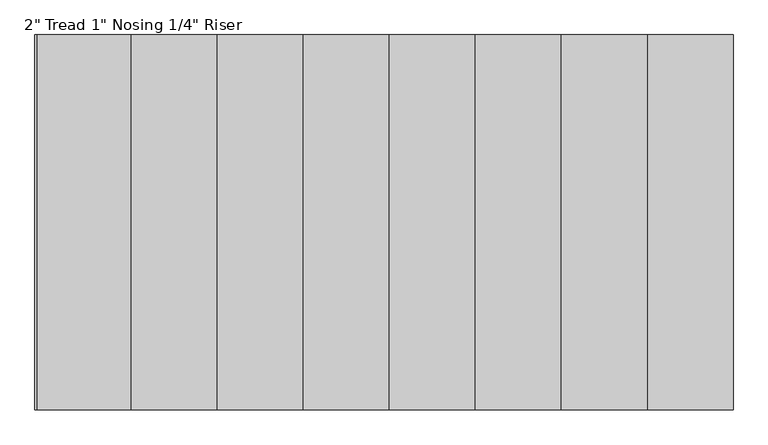
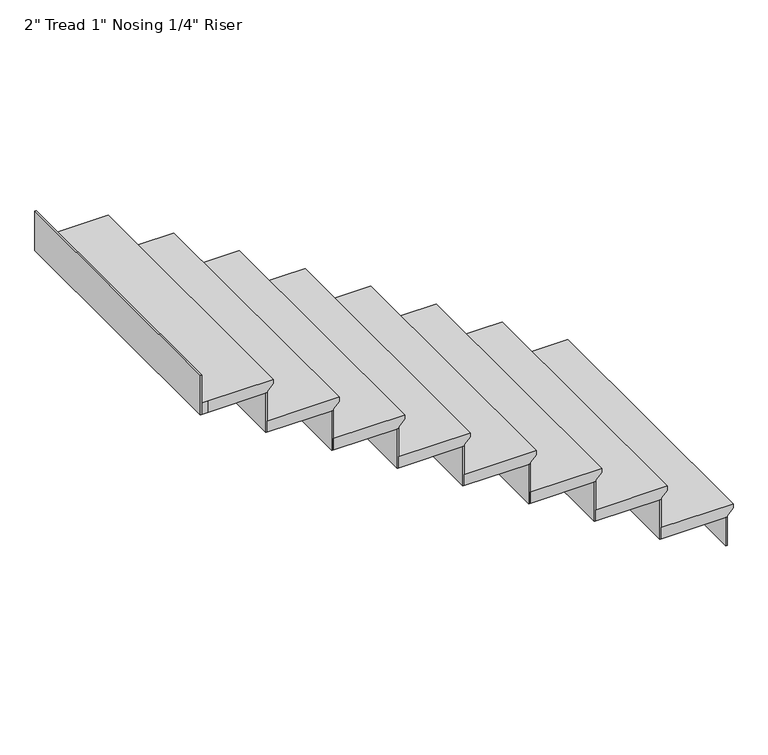
"""IFC4 building model written with IfcOpenShell, lengths in millimetres: stair flight geometry."""

from ifc_helpers import new_model, si_unit, origin, place, context, project, spatial, faceted_brep, source, transform, mapped, element, save


def stair_flight_d31f5684(model_context):
    return source(origin(), model_context, "Body", "Brep", [
        faceted_brep([(-5888.2707895, 6233.3144188, 3359.15), (-5888.2707895, 6233.3144188, 3378.2), (-5888.2707895, 5014.1144188, 3378.2), (-5888.2707895, 5014.1144188, 3359.15), (-5913.6707895, 6233.3144188, 3333.75), (-5913.6707895, 5014.1144188, 3333.75), (-6193.0707895, 6233.3144188, 3378.2), (-6193.0707895, 5014.1144188, 3378.2), (-5913.6707895, 5014.1144188, 3327.4), (-6193.0707895, 5014.1144188, 3327.4), (-6193.0707895, 6233.3144188, 3327.4), (-5913.6707895, 6233.3144188, 3327.4)], [[[0, 1, 2, 3]], [[4, 0, 3, 5]], [[2, 1, 6, 7]], [[8, 9, 10, 11]], [[2, 7, 9, 8, 5, 3]], [[8, 11, 4, 5]], [[6, 1, 0, 4, 11, 10]], [[7, 6, 10, 9]]]),
        faceted_brep([(-5913.6707895, 6233.3144188, 3327.4), (-5913.6707895, 6233.3144188, 3200.4), (-5920.0207895, 6233.3144188, 3200.4), (-5920.0207895, 6233.3144188, 3327.4), (-5913.6707895, 5014.1144188, 3327.4), (-5920.0207895, 5014.1144188, 3327.4), (-5920.0207895, 5014.1144188, 3200.4), (-5913.6707895, 5014.1144188, 3200.4)], [[[0, 1, 2, 3]], [[4, 5, 6, 7]], [[1, 0, 4, 7]], [[2, 1, 7, 6]], [[3, 2, 6, 5]], [[0, 3, 5, 4]]]),
        faceted_brep([(-6193.0707895, 6233.3144188, 3505.2), (-6193.0707895, 6233.3144188, 3327.4), (-6199.4207895, 6233.3144188, 3327.4), (-6199.4207895, 6233.3144188, 3505.2), (-6193.0707895, 5014.1144188, 3505.2), (-6199.4207895, 5014.1144188, 3505.2), (-6199.4207895, 5014.1144188, 3327.4), (-6193.0707895, 5014.1144188, 3327.4)], [[[0, 1, 2, 3]], [[4, 5, 6, 7]], [[1, 0, 4, 7]], [[2, 1, 7, 6]], [[3, 2, 6, 5]], [[0, 3, 5, 4]]]),
        faceted_brep([(-6167.6707895, 5014.1144188, 3556.0), (-6167.6707895, 6233.3144188, 3556.0), (-6472.4707895, 6233.3144188, 3556.0), (-6472.4707895, 5014.1144188, 3556.0), (-6193.0707895, 5014.1144188, 3505.2), (-6472.4707895, 5014.1144188, 3505.2), (-6472.4707895, 6233.3144188, 3505.2), (-6193.0707895, 6233.3144188, 3505.2), (-6193.0707895, 5014.1144188, 3511.55), (-6167.6707895, 5014.1144188, 3536.95), (-6193.0707895, 6233.3144188, 3511.55), (-6167.6707895, 6233.3144188, 3536.95)], [[[0, 1, 2, 3]], [[4, 5, 6, 7]], [[0, 3, 5, 4, 8, 9]], [[4, 7, 10, 8]], [[2, 1, 11, 10, 7, 6]], [[3, 2, 6, 5]], [[11, 1, 0, 9]], [[10, 11, 9, 8]]]),
        faceted_brep([(-6472.4707895, 6233.3144188, 3683.0), (-6472.4707895, 6233.3144188, 3505.2), (-6478.8207895, 6233.3144188, 3505.2), (-6478.8207895, 6233.3144188, 3683.0), (-6472.4707895, 5014.1144188, 3683.0), (-6478.8207895, 5014.1144188, 3683.0), (-6478.8207895, 5014.1144188, 3505.2), (-6472.4707895, 5014.1144188, 3505.2)], [[[0, 1, 2, 3]], [[4, 5, 6, 7]], [[1, 0, 4, 7]], [[2, 1, 7, 6]], [[3, 2, 6, 5]], [[0, 3, 5, 4]]]),
        faceted_brep([(-6447.0707895, 5014.1144188, 3733.8), (-6447.0707895, 6233.3144188, 3733.8), (-6751.8707895, 6233.3144188, 3733.8), (-6751.8707895, 5014.1144188, 3733.8), (-6472.4707895, 5014.1144188, 3683.0), (-6751.8707895, 5014.1144188, 3683.0), (-6751.8707895, 6233.3144188, 3683.0), (-6472.4707895, 6233.3144188, 3683.0), (-6472.4707895, 5014.1144188, 3689.35), (-6447.0707895, 5014.1144188, 3714.75), (-6472.4707895, 6233.3144188, 3689.35), (-6447.0707895, 6233.3144188, 3714.75)], [[[0, 1, 2, 3]], [[4, 5, 6, 7]], [[0, 3, 5, 4, 8, 9]], [[4, 7, 10, 8]], [[2, 1, 11, 10, 7, 6]], [[3, 2, 6, 5]], [[11, 1, 0, 9]], [[10, 11, 9, 8]]]),
        faceted_brep([(-6751.8707895, 6233.3144188, 3860.8), (-6751.8707895, 6233.3144188, 3683.0), (-6758.2207895, 6233.3144188, 3683.0), (-6758.2207895, 6233.3144188, 3860.8), (-6751.8707895, 5014.1144188, 3860.8), (-6758.2207895, 5014.1144188, 3860.8), (-6758.2207895, 5014.1144188, 3683.0), (-6751.8707895, 5014.1144188, 3683.0)], [[[0, 1, 2, 3]], [[4, 5, 6, 7]], [[1, 0, 4, 7]], [[2, 1, 7, 6]], [[3, 2, 6, 5]], [[0, 3, 5, 4]]]),
        faceted_brep([(-6726.4707895, 5014.1144188, 3911.6), (-6726.4707895, 6233.3144188, 3911.6), (-7031.2707895, 6233.3144188, 3911.6), (-7031.2707895, 5014.1144188, 3911.6), (-6751.8707895, 5014.1144188, 3860.8), (-7031.2707895, 5014.1144188, 3860.8), (-7031.2707895, 6233.3144188, 3860.8), (-6751.8707895, 6233.3144188, 3860.8), (-6751.8707895, 5014.1144188, 3867.15), (-6726.4707895, 5014.1144188, 3892.55), (-6751.8707895, 6233.3144188, 3867.15), (-6726.4707895, 6233.3144188, 3892.55)], [[[0, 1, 2, 3]], [[4, 5, 6, 7]], [[0, 3, 5, 4, 8, 9]], [[4, 7, 10, 8]], [[2, 1, 11, 10, 7, 6]], [[3, 2, 6, 5]], [[11, 1, 0, 9]], [[10, 11, 9, 8]]]),
        faceted_brep([(-7031.2707895, 6233.3144188, 4038.6), (-7031.2707895, 6233.3144188, 3860.8), (-7037.6207895, 6233.3144188, 3860.8), (-7037.6207895, 6233.3144188, 4038.6), (-7031.2707895, 5014.1144188, 4038.6), (-7037.6207895, 5014.1144188, 4038.6), (-7037.6207895, 5014.1144188, 3860.8), (-7031.2707895, 5014.1144188, 3860.8)], [[[0, 1, 2, 3]], [[4, 5, 6, 7]], [[1, 0, 4, 7]], [[2, 1, 7, 6]], [[3, 2, 6, 5]], [[0, 3, 5, 4]]]),
        faceted_brep([(-7005.8707895, 5014.1144188, 4089.4), (-7005.8707895, 6233.3144188, 4089.4), (-7310.6707895, 6233.3144188, 4089.4), (-7310.6707895, 5014.1144188, 4089.4), (-7031.2707895, 5014.1144188, 4038.6), (-7310.6707895, 5014.1144188, 4038.6), (-7310.6707895, 6233.3144188, 4038.6), (-7031.2707895, 6233.3144188, 4038.6), (-7031.2707895, 5014.1144188, 4044.95), (-7005.8707895, 5014.1144188, 4070.35), (-7031.2707895, 6233.3144188, 4044.95), (-7005.8707895, 6233.3144188, 4070.35)], [[[0, 1, 2, 3]], [[4, 5, 6, 7]], [[0, 3, 5, 4, 8, 9]], [[4, 7, 10, 8]], [[2, 1, 11, 10, 7, 6]], [[3, 2, 6, 5]], [[11, 1, 0, 9]], [[10, 11, 9, 8]]]),
        faceted_brep([(-7310.6707895, 6233.3144188, 4216.4), (-7310.6707895, 6233.3144188, 4038.6), (-7317.0207895, 6233.3144188, 4038.6), (-7317.0207895, 6233.3144188, 4216.4), (-7310.6707895, 5014.1144188, 4216.4), (-7317.0207895, 5014.1144188, 4216.4), (-7317.0207895, 5014.1144188, 4038.6), (-7310.6707895, 5014.1144188, 4038.6)], [[[0, 1, 2, 3]], [[4, 5, 6, 7]], [[1, 0, 4, 7]], [[2, 1, 7, 6]], [[3, 2, 6, 5]], [[0, 3, 5, 4]]]),
        faceted_brep([(-7285.2707895, 5014.1144188, 4267.2), (-7285.2707895, 6233.3144188, 4267.2), (-7590.0707895, 6233.3144188, 4267.2), (-7590.0707895, 5014.1144188, 4267.2), (-7310.6707895, 5014.1144188, 4216.4), (-7590.0707895, 5014.1144188, 4216.4), (-7590.0707895, 6233.3144188, 4216.4), (-7310.6707895, 6233.3144188, 4216.4), (-7310.6707895, 5014.1144188, 4222.75), (-7285.2707895, 5014.1144188, 4248.15), (-7310.6707895, 6233.3144188, 4222.75), (-7285.2707895, 6233.3144188, 4248.15)], [[[0, 1, 2, 3]], [[4, 5, 6, 7]], [[0, 3, 5, 4, 8, 9]], [[4, 7, 10, 8]], [[2, 1, 11, 10, 7, 6]], [[3, 2, 6, 5]], [[11, 1, 0, 9]], [[10, 11, 9, 8]]]),
        faceted_brep([(-7590.0707895, 6233.3144188, 4394.2), (-7590.0707895, 6233.3144188, 4216.4), (-7596.4207895, 6233.3144188, 4216.4), (-7596.4207895, 6233.3144188, 4394.2), (-7590.0707895, 5014.1144188, 4394.2), (-7596.4207895, 5014.1144188, 4394.2), (-7596.4207895, 5014.1144188, 4216.4), (-7590.0707895, 5014.1144188, 4216.4)], [[[0, 1, 2, 3]], [[4, 5, 6, 7]], [[1, 0, 4, 7]], [[2, 1, 7, 6]], [[3, 2, 6, 5]], [[0, 3, 5, 4]]]),
        faceted_brep([(-7564.6707895, 5014.1144188, 4445.0), (-7564.6707895, 6233.3144188, 4445.0), (-7869.4707895, 6233.3144188, 4445.0), (-7869.4707895, 5014.1144188, 4445.0), (-7590.0707895, 5014.1144188, 4394.2), (-7869.4707895, 5014.1144188, 4394.2), (-7869.4707895, 6233.3144188, 4394.2), (-7590.0707895, 6233.3144188, 4394.2), (-7590.0707895, 5014.1144188, 4400.55), (-7564.6707895, 5014.1144188, 4425.95), (-7590.0707895, 6233.3144188, 4400.55), (-7564.6707895, 6233.3144188, 4425.95)], [[[0, 1, 2, 3]], [[4, 5, 6, 7]], [[0, 3, 5, 4, 8, 9]], [[4, 7, 10, 8]], [[2, 1, 11, 10, 7, 6]], [[3, 2, 6, 5]], [[11, 1, 0, 9]], [[10, 11, 9, 8]]]),
        faceted_brep([(-8148.8707895, 6233.3144188, 4749.8), (-8148.8707895, 6233.3144188, 4572.0), (-8155.2207895, 6233.3144188, 4572.0), (-8155.2207895, 6233.3144188, 4749.8), (-8148.8707895, 5014.1144188, 4749.8), (-8155.2207895, 5014.1144188, 4749.8), (-8155.2207895, 5014.1144188, 4572.0), (-8148.8707895, 5014.1144188, 4572.0)], [[[0, 1, 2, 3]], [[4, 5, 6, 7]], [[1, 0, 4, 7]], [[2, 1, 7, 6]], [[3, 2, 6, 5]], [[0, 3, 5, 4]]]),
        faceted_brep([(-7869.4707895, 6233.3144188, 4572.0), (-7869.4707895, 6233.3144188, 4394.2), (-7875.8207895, 6233.3144188, 4394.2), (-7875.8207895, 6233.3144188, 4572.0), (-7869.4707895, 5014.1144188, 4572.0), (-7875.8207895, 5014.1144188, 4572.0), (-7875.8207895, 5014.1144188, 4394.2), (-7869.4707895, 5014.1144188, 4394.2)], [[[0, 1, 2, 3]], [[4, 5, 6, 7]], [[1, 0, 4, 7]], [[2, 1, 7, 6]], [[3, 2, 6, 5]], [[0, 3, 5, 4]]]),
        faceted_brep([(-8148.8707895, 5014.1144188, 4622.8), (-8123.4707895, 5014.1144188, 4622.8), (-7844.0707895, 5014.1144188, 4622.8), (-7844.0707895, 6233.3144188, 4622.8), (-8148.8707895, 6233.3144188, 4622.8), (-8123.4707895, 5014.1144188, 4572.0), (-8148.8707895, 5014.1144188, 4572.0), (-8148.8707895, 6233.3144188, 4572.0), (-7869.4707895, 6233.3144188, 4572.0), (-7869.4707895, 5014.1144188, 4572.0), (-7869.4707895, 5014.1144188, 4578.35), (-7844.0707895, 5014.1144188, 4603.75), (-7869.4707895, 6233.3144188, 4578.35), (-7844.0707895, 6233.3144188, 4603.75)], [[[0, 1, 2, 3, 4]], [[5, 6, 7, 8, 9]], [[1, 0, 6, 5]], [[2, 1, 5, 9, 10, 11]], [[9, 8, 12, 10]], [[4, 3, 13, 12, 8, 7]], [[0, 4, 7, 6]], [[13, 3, 2, 11]], [[12, 13, 11, 10]]]),
    ])


if __name__ == "__main__":
    model = new_model("IFC4")
    model_context = context("Model", 3, world=origin())
    ifc_project = project(units=[si_unit("LENGTHUNIT", "METRE", prefix="MILLI")], contexts=[model_context])
    site = spatial("IfcSite", under=ifc_project)
    building = spatial("IfcBuilding", under=site)
    placement = place(None, origin())
    stair_flight_shape = stair_flight_d31f5684(model_context)
    element("IfcStairFlight", 1, ObjectType="2\" Tread 1\" Nosing 1/4\" Riser", at=placement, inside=building, context=model_context, shape_type="MappedRepresentation", body=[
        mapped(stair_flight_shape, transform((0.0, 0.0, 0.0), x_axis=(1.0, 0.0, 0.0), y_axis=(0.0, 1.0, 0.0), z_axis=(0.0, 0.0, 1.0))),
    ])
    save(model, "model.ifc")
